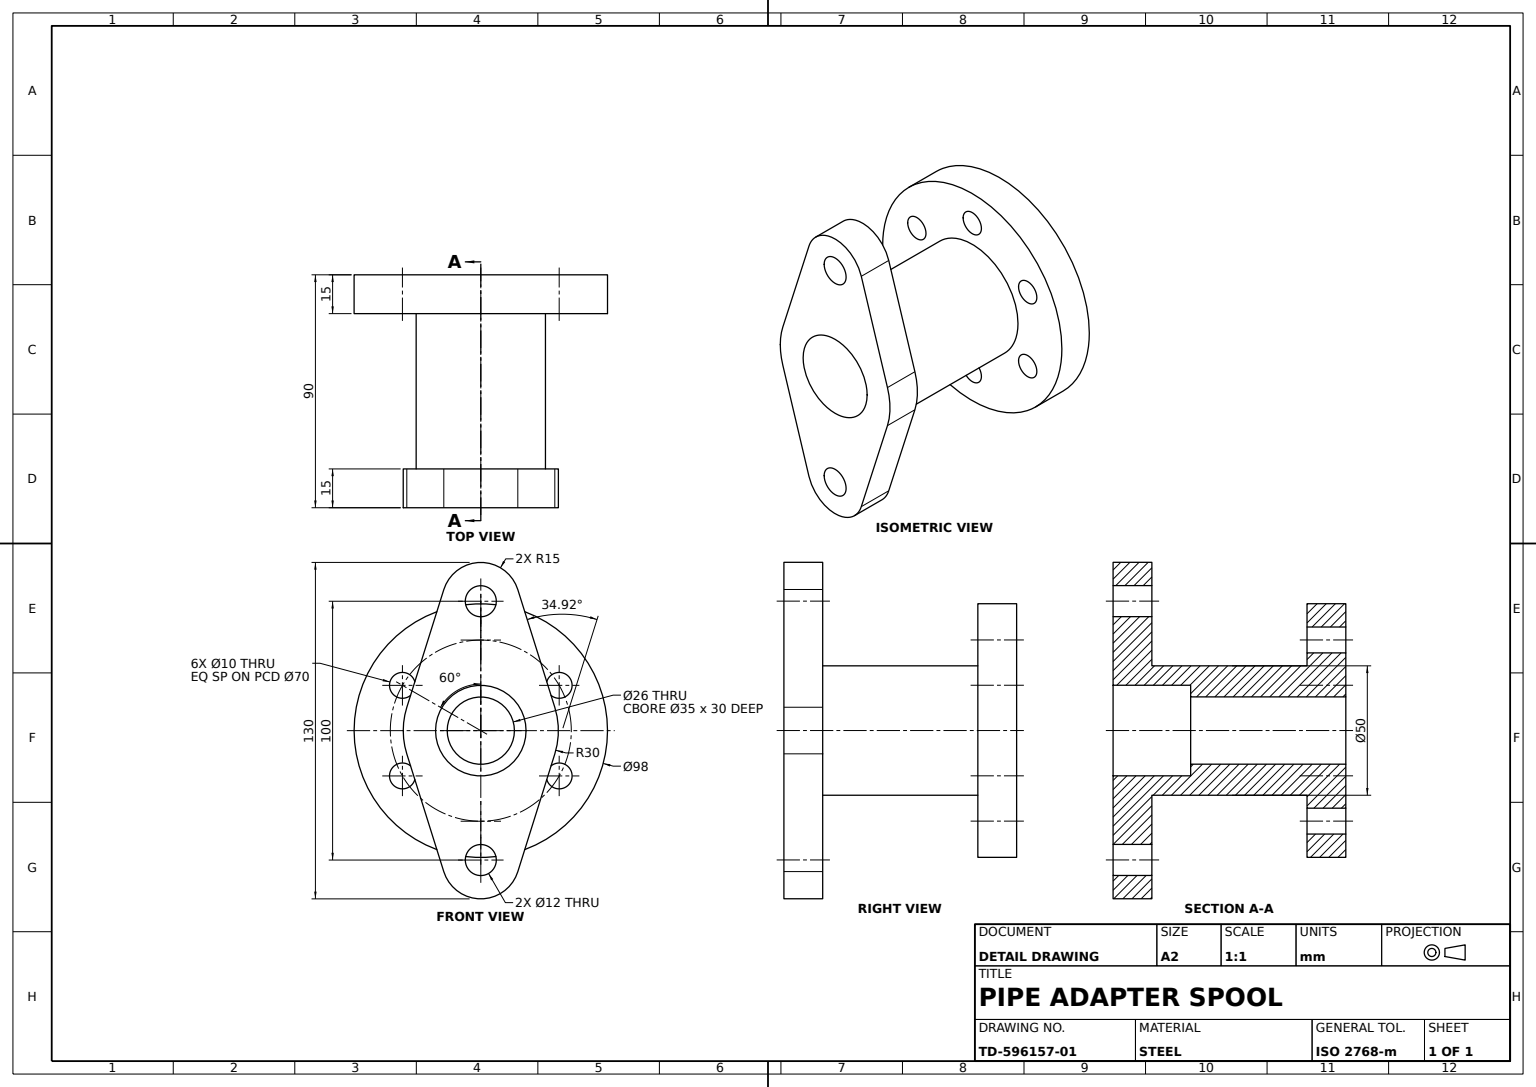
SolidWorks part; units mm, degrees
material "Plain Carbon Steel"
ref_plane "Front Plane" through (0, 0, 0) normal (0, 0, 1) x (1, 0, 0)
ref_plane "Top Plane" through (0, 0, 0) normal (0, 1, 0) x (1, 0, 0)
ref_plane "Right Plane" through (0, 0, 0) normal (1, 0, 0) x (0, 0, -1)
sketch "Round Flange Sketch" plane through (0, 0, 0) normal (0, 0, 1) x (1, 0, 0)
  circle A0 centre (0, 0) radius 49
  circle A2 centre (0, 0) radius 13
  circle A3 centre (0, 35) radius 5
  circle A4 centre (30.3109, 17.5) radius 5
  circle A5 centre (30.3109, -17.5) radius 5
  circle A6 centre (0, -35) radius 5
  circle A7 centre (-30.3109, -17.5) radius 5
  circle A8 centre (-30.3109, 17.5) radius 5
  dimension "D1" = 98
  dimension "D2" = 35
  dimension "D3" = 26
  dimension "D4" = 10
  dimension "D6" = 30.3109
  dimension "D7" = 17.5
  dimension "D5" = 6
extrude "Round Flange Ø98 6xØ10" add sketch "Round Flange Sketch" along normal blind 15
sketch "Tube Sketch" plane through (0, 0, 15) normal (0, 0, 1) x (1, 0, 0)
  circle A0 centre (0, 0) radius 13
  circle A1 centre (0, 0) radius 25
  dimension "D1" = 50
  dimension "D2" = 26
extrude "Tube Ø50 Bore Ø26" add sketch "Tube Sketch" along normal blind 45
sketch "Collar Sketch" plane through (0, 0, 60) normal (0, 0, 1) x (1, 0, 0)
  circle A0 centre (0, 0) radius 17.5
  circle A1 centre (0, 0) radius 25
  dimension "D1" = 35
  dimension "D2" = 50
extrude "Collar" add sketch "Collar Sketch" along normal blind 15
sketch "Oval Flange Sketch" plane through (0, 0, 75) normal (0, 0, 1) x (1, 0, 0)
  line L0 (-28.6182, 9) -> (-14.3091, 54.5)
  line L1 (28.6182, 9) -> (14.3091, 54.5)
  line L2 (-28.6182, -9) -> (-14.3091, -54.5)
  line L3 (28.6182, -9) -> (14.3091, -54.5)
  circle A0 centre (0, 50) radius 15
  circle A1 centre (0, 50) radius 6
  circle A2 centre (0, -50) radius 6
  circle A3 centre (0, -50) radius 15
  arc A4 (-28.6182, 9) -> (-28.6182, -9) centre (0, 0) ccw
  circle A5 centre (0, 0) radius 17.5
  arc A6 (28.6182, -9) -> (28.6182, 9) centre (0, 0) ccw
  circle M5 centre (0, 0) radius 25
  circle M6 centre (0, 0) radius 17.5
  dimension "D1" = 30
  dimension "D2" = 12
  dimension "D3" = 12
  dimension "D4" = 30
  dimension "D8" = 60
  dimension "D9" = 35
  dimension "D5" = 50
  dimension "D6" = 50
  dimension "D7" = 100
  dimension "D10" = 28.6182
extrude "Oval Flange 2xØ12" add sketch "Oval Flange Sketch" along normal blind 15 contours L3 A6 L1 A0 L0 A4 L2 A3 M5 | M5 M6 | A0 A1 | A3 A2
